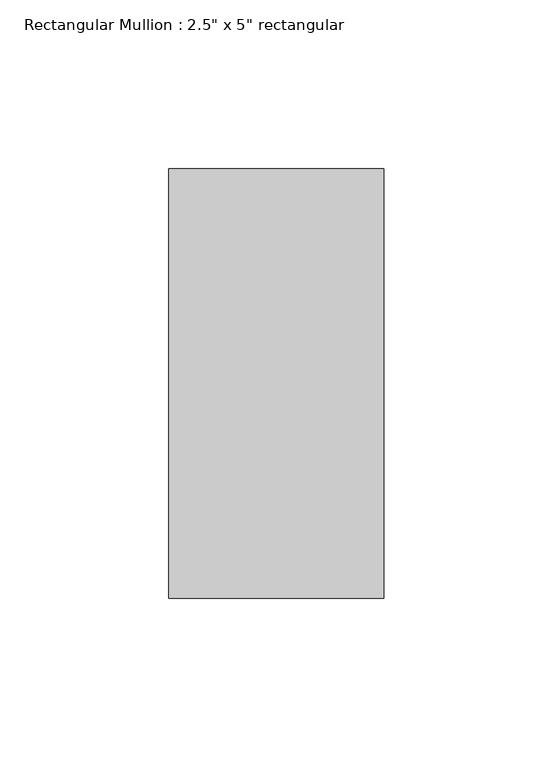
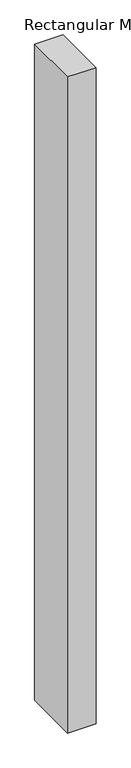
"""IFC4 building model written with IfcOpenShell, lengths in millimetres: member geometry."""

from ifc_helpers import new_model, si_unit, frame, origin, place, context, project, spatial, polyline, outline, extrude, source, transform, mapped, element, save


def member_c1df12fd(model_context):
    return source(origin(), model_context, "Body", "SweptSolid", [
        extrude(outline(polyline([(31.75, 63.5), (31.75, -63.5), (-31.75, -63.5), (-31.75, 63.5), (31.75, 63.5)])), frame((0.0, 0.0, -1549.4), z_axis=(0.0, 0.0, 1.0), x_axis=(1.0, 0.0, 0.0)), (0.0, 0.0, 1.0), 1549.4),
    ])


if __name__ == "__main__":
    model = new_model("IFC4")
    model_context = context("Model", 3, world=origin())
    ifc_project = project(units=[si_unit("LENGTHUNIT", "METRE", prefix="MILLI")], contexts=[model_context])
    site = spatial("IfcSite", under=ifc_project)
    building = spatial("IfcBuilding", under=site)
    placement = place(None, origin())
    member_shape = member_c1df12fd(model_context)
    element("IfcMember", 1, ObjectType="Rectangular Mullion : 2.5\" x 5\" rectangular", at=placement, inside=building, context=model_context, shape_type="MappedRepresentation", body=[
        mapped(member_shape, transform((0.0, 0.0, 0.0), x_axis=(1.0, 0.0, 0.0), y_axis=(0.0, 1.0, 0.0), z_axis=(0.0, 0.0, 1.0))),
    ])
    save(model, "model.ifc")

# Revit data of these elements
# Type "Rectangular Mullion : 2.5\" x 5\" rectangular"
#   built-in parameter 1007304 = 0.416667 (stored number, unit not read)
#   built-in parameter 1007301 = 0.104167 (stored number, unit not read)
#   built-in parameter 1007300 = 0.104167 (stored number, unit not read)
